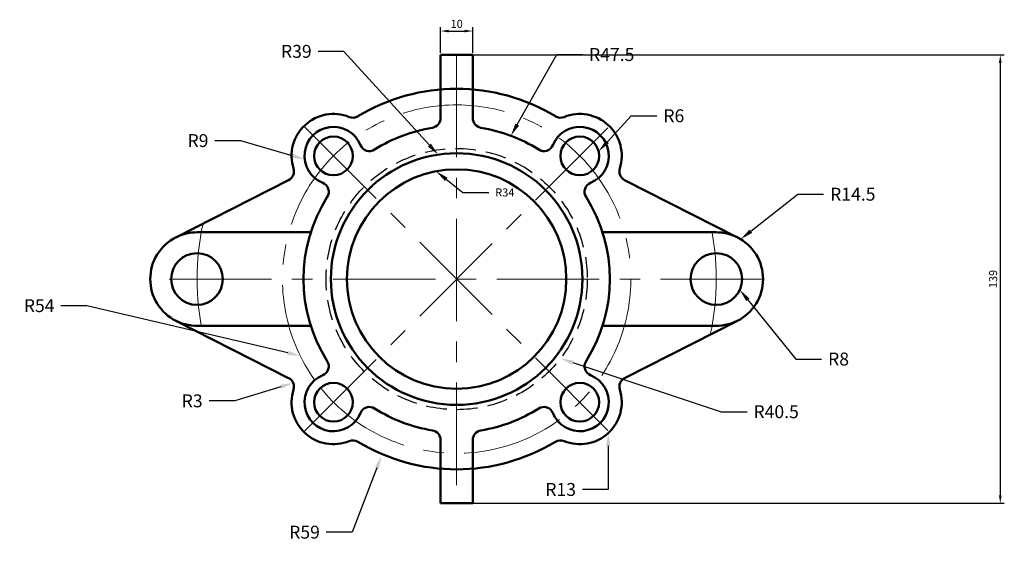
# Model space of a CAD drawing. Units: millimetres. Extents: x 2698 to 3004, y 1503 to 1665.
import ezdxf
from ezdxf import colors
from ezdxf.entities.mleader import LeaderData, LeaderLine
from ezdxf.math import Vec2, Vec3

# ---------------------------------------------------------------- set-up
doc = ezdxf.new("R2010")
doc.units = ezdxf.units.MM
doc.linetypes.add('CENTER', pattern=[50.8, 31.75, -6.35, 6.35, -6.35])
doc.linetypes.add('HIDDEN', pattern=[9.525, 6.35, -3.175])
for name, color, linetype, lineweight in [('M-CNTR', 4, 'CENTER', 18), ('M-DIMS', 2, 'Continuous', 25), ('M-HIDN', 1, 'HIDDEN', 25), ('M-OUTL', 7, 'Continuous', 50), ('M-TEXT', 3, 'Continuous', 25)]:
    doc.layers.add(name, color=color, linetype=linetype, lineweight=lineweight)
doc.styles.get("Standard").update_dxf_attribs({"font": 'arial.ttf'})
doc.dimstyles.new('ISO-25', dxfattribs={"dimtxt": 2.5, "dimasz": 2.5, "dimexe": 1.25, "dimexo": 0.625, "dimtad": 1, "dimtxsty": 'Standard', "dimcen": 2.5, "dimadec": 0, "dimazin": 0, "dimtfac": 1, "dimtmove": 0, "dimatfit": 3, "dimfxl": 1, "dimarcsym": 0})

# ---------------------------------------------------------------- blocks, each defined once
blk = doc.blocks.new('*D1')
at = {"layer": 'Defpoints', "color": 0, "transparency": 16777216}
for p in [(2838.92, 1661.31), (2828.92, 1653.93), (2838.92, 1653.93)]:
    blk.add_point(p, dxfattribs=at)
at = {"layer": 'M-DIMS', "color": 0, "lineweight": -2, "transparency": 16777216}
for p, q in [((2828.92, 1654.55), (2828.92, 1662.56)), ((2831.42, 1661.31), (2836.42, 1661.31)), ((2838.92, 1654.55), (2838.92, 1662.56))]:
    blk.add_line(p, q, dxfattribs=at)
at = {"layer": 'M-DIMS', "color": 0, "transparency": 16777216}
for points in [[(2831.42, 1661.72), (2831.42, 1660.89), (2828.92, 1661.31)], [(2836.42, 1661.72), (2836.42, 1660.89), (2838.92, 1661.31)]]:
    blk.add_solid(points, dxfattribs=at)
at = {"layer": 'M-DIMS', "color": 0, "transparency": 16777216, "insert": (2833.92, 1663.21), "char_height": 2.5, "attachment_point": 5}
blk.add_mtext('10', dxfattribs=at)
blk = doc.blocks.new('*D2')
at = {"layer": 'Defpoints', "color": 0, "transparency": 16777216}
for p in [(2833.92, 1653.93), (2833.92, 1514.93), (3002.46, 1514.93)]:
    blk.add_point(p, dxfattribs=at)
at = {"layer": 'M-DIMS', "color": 0, "lineweight": -2, "transparency": 16777216}
for p, q in [((2834.54, 1653.93), (3003.71, 1653.93)), ((3002.46, 1651.43), (3002.46, 1517.43)), ((2834.54, 1514.93), (3003.71, 1514.93))]:
    blk.add_line(p, q, dxfattribs=at)
at = {"layer": 'M-DIMS', "color": 0, "transparency": 16777216}
for points in [[(3002.04, 1651.43), (3002.87, 1651.43), (3002.46, 1653.93)], [(3002.04, 1517.43), (3002.87, 1517.43), (3002.46, 1514.93)]]:
    blk.add_solid(points, dxfattribs=at)
at = {"layer": 'M-DIMS', "color": 0, "transparency": 16777216, "insert": (3000.56, 1584.43), "char_height": 2.5, "attachment_point": 5, "rotation": 90}
blk.add_mtext('139', dxfattribs=at)
blk = doc.blocks.new('BOLT-HOLE-LUG')
blk.add_circle((12.73, 8.61), 6)
blk.add_arc((12.73, 8.61), 9, 21.8384, 248.1616)

msp = doc.modelspace()

# ---------------------------------------------------------------- linework, layer by layer
at = {"layer": 'M-CNTR'}
for p, q in [((2833.916, 1653.928), (2833.916, 1514.928)), ((2786.54, 1537.052), (2881.292, 1631.804)), ((2786.54, 1631.804), (2881.292, 1537.052)), ((2928.916, 1584.428), (2738.916, 1584.428))]:
    msp.add_line(p, q, dxfattribs=at)
for radius, start, end in [(54, 218.63053, 215.43962), (80.5, 167.65726, 192.34274), (80.5, 347.65726, 12.34274)]:
    msp.add_arc((2833.916, 1584.428), radius, start, end, dxfattribs=at)
at = {"layer": 'M-HIDN'}
msp.add_circle((2833.916, 1584.428), 40.5, dxfattribs=at)
at = {"layer": 'M-OUTL'}
for p, q in [((2828.916, 1653.928), (2838.916, 1653.928)), ((2828.916, 1634.29), (2828.916, 1653.928)), ((2838.916, 1653.928), (2838.916, 1634.29)), ((2746.85, 1597.356), (2781.832, 1615.122)), ((2920.982, 1597.356), (2886, 1615.122)), ((2753.416, 1598.928), (2788.683, 1598.928)), ((2879.149, 1598.928), (2914.416, 1598.928)), ((2746.85, 1571.499), (2781.832, 1553.734)), ((2753.416, 1569.928), (2788.683, 1569.928)), ((2879.149, 1569.928), (2914.416, 1569.928)), ((2920.982, 1571.499), (2886, 1553.734)), ((2828.916, 1534.565), (2828.916, 1514.928)), ((2838.916, 1534.565), (2838.916, 1514.928)), ((2838.916, 1514.928), (2828.916, 1514.928))]:
    msp.add_line(p, q, dxfattribs=at)
for centre, radius in [((2833.916, 1584.428), 39), ((2833.916, 1584.428), 34), ((2753.416, 1584.428), 8), ((2914.416, 1584.428), 8)]:
    msp.add_circle(centre, radius, dxfattribs=at)
for centre, radius, start, end in [((2833.916, 1584.428), 59, 58.75383, 121.24617), ((2795.732, 1622.612), 13, 67.88538, 197.51435), ((2801.756, 1637.434), 3, 247.88538, 301.24617), ((2825.916, 1634.29), 3, 279.11496, 0), ((2841.916, 1634.29), 3, 180, 260.88504), ((2866.076, 1637.434), 3, 238.75383, 292.11462), ((2872.1, 1622.612), 13, 342.48565, 112.11462), ((2833.916, 1584.428), 47.5, 99.11496, 122.38075), ((2833.916, 1584.428), 47.5, 57.61925, 80.88504), ((2806.871, 1627.075), 3, 201.83841, 302.38075), ((2860.961, 1627.075), 3, 237.61925, 338.16159), ((2780.474, 1617.796), 3, 296.92354, 17.51435), ((2887.358, 1617.796), 3, 162.48565, 243.07646), ((2791.268, 1611.473), 3, 327.61925, 68.16159), ((2876.564, 1611.473), 3, 111.83841, 212.38075), ((2833.916, 1584.428), 47.5, 147.61925, 212.38075), ((2833.916, 1584.428), 47.5, 327.61925, 32.38075), ((2753.416, 1584.428), 14.5, 84.83282, 275.16718), ((2914.416, 1584.428), 14.5, 264.83282, 95.16718), ((2791.268, 1557.383), 3, 291.83841, 32.38075), ((2876.564, 1557.383), 3, 147.61925, 248.16159), ((2780.474, 1551.059), 3, 342.48565, 63.07646), ((2887.358, 1551.059), 3, 116.92354, 197.51435), ((2795.732, 1546.244), 13, 162.48565, 292.11462), ((2872.1, 1546.244), 13, 247.88538, 17.51435), ((2806.871, 1541.78), 3, 57.61925, 158.16159), ((2860.961, 1541.78), 3, 21.83841, 122.38075), ((2833.916, 1584.428), 47.5, 237.61925, 260.88504), ((2833.916, 1584.428), 47.5, 279.11496, 302.38075), ((2825.916, 1534.565), 3, 0, 80.88504), ((2841.916, 1534.565), 3, 99.11496, 180), ((2801.756, 1531.421), 3, 58.75383, 112.11462), ((2833.916, 1584.428), 59, 238.75383, 301.24617), ((2866.076, 1531.421), 3, 67.88538, 121.24617)]:
    msp.add_arc(centre, radius, start, end, dxfattribs=at)

# ---------------------------------------------------------------- block references
msp.add_blockref('BOLT-HOLE-LUG', (2783, 1614), dxfattribs=at)
for p, rotation in [((2863.488, 1635.344), 270.0000000000005), ((2804.344, 1533.512), 90.00000000000315), ((2884.832, 1554.856), 180)]:
    msp.add_blockref('BOLT-HOLE-LUG', p, dxfattribs=dict(at, rotation=rotation))

# ---------------------------------------------------------------- dimensions: what is measured, and where the dimension line sits
at = {"layer": 'M-DIMS'}
dim = msp.add_linear_dim(base=(2838.916, 1661.307), p1=(2828.916, 1653.928), p2=(2838.916, 1653.928), dimstyle='ISO-25', override={"dimclrd": 0, "dimclre": 0, "dimclrt": 0}, dxfattribs=at)
dim.commit()
dim.dimension.update_dxf_attribs({"geometry": '*D1', "text_midpoint": (2833.916, 1663.209)})
dim = msp.add_linear_dim(base=(3002.458, 1514.928), p1=(2833.916, 1653.928), p2=(2833.916, 1514.928), angle=90, dimstyle='ISO-25', override={"dimclrd": 0, "dimclre": 0, "dimclrt": 0}, dxfattribs=at)
dim.commit()
dim.dimension.update_dxf_attribs({"geometry": '*D2', "text_midpoint": (3000.556, 1584.428)})

# ---------------------------------------------------------------- leaders
at = {"layer": 'M-TEXT'}
ml = msp.add_multileader_mtext('Standard', dxfattribs=at)
ml.set_content('R39', color=256)
ml.set_leader_properties()
ml.build(insert=Vec2(0, 0))
ctx = ml.context
ctx.base_point, ctx.plane_origin = Vec3(2777.405, 1654.98), Vec3(2828.164, 1623.001)
ctx.text_align_type = 2
notes = []
notes.append((ctx, [(0, (1, 1, 0), (2798.972, 1654.98), (-1, 0), 8, [(0, [(2828.164, 1623.001)], 0, [])])]))
ctx.mtext.insert, ctx.mtext.alignment, ctx.mtext.flow_direction = Vec3(2788.972, 1657.015), 3, 5
ml = msp.add_multileader_mtext('Standard', dxfattribs=at)
ml.set_content('R47.5', color=256)
ml.set_leader_properties()
ml.build(insert=Vec2(0, 0))
ctx = ml.context
ctx.base_point, ctx.plane_origin = Vec3(2872.956, 1653.993), Vec3(2850.743, 1628.847)
notes.append((ctx, [(0, (1, 1, 0), (2864.956, 1653.993), (1, 0), 8, [(0, [(2850.743, 1628.847)], 0, [])])]))
ctx.mtext.insert, ctx.mtext.flow_direction = Vec3(2874.956, 1656.027), 5
ml = msp.add_multileader_mtext('Standard', dxfattribs=at)
ml.set_content('R6', color=256)
ml.set_leader_properties()
ml.build(insert=Vec2(0, 0))
ctx = ml.context
ctx.base_point, ctx.plane_origin = Vec3(2896, 1635.013), Vec3(2877.935, 1624.008)
notes.append((ctx, [(0, (1, 1, 0), (2888, 1635.013), (1, 0), 8, [(0, [(2877.935, 1624.008)], 0, [])])]))
ctx.mtext.insert, ctx.mtext.flow_direction = Vec3(2898, 1637.047), 5
ml = msp.add_multileader_mtext('Standard', dxfattribs=at)
ml.set_content('R9', color=256)
ml.set_leader_properties()
ml.build(insert=Vec2(0, 0))
ctx = ml.context
ctx.base_point, ctx.plane_origin = Vec3(2748.509, 1627.319), Vec3(2786.796, 1621.538)
ctx.text_align_type = 2
notes.append((ctx, [(0, (1, 1, 0), (2766.968, 1627.319), (-1, 0), 8, [(0, [(2786.796, 1621.538)], 0, [])])]))
ctx.mtext.insert, ctx.mtext.alignment, ctx.mtext.flow_direction = Vec3(2756.968, 1629.353), 3, 5
ml = msp.add_multileader_mtext('Standard', dxfattribs=at)
ml.set_content('R34', color=256)
ml.set_leader_properties()
ml.build(insert=Vec2(0, 0))
ctx = ml.context
ctx.base_point, ctx.char_height, ctx.plane_origin = Vec3(2843.883, 1611.259), 2.5, Vec3(2827.54, 1617.825)
notes.append((ctx, [(0, (1, 1, 0), (2835.883, 1611.259), (1, 0), 8, [(0, [(2827.54, 1617.825)], 0, [])])]))
ctx.mtext.insert, ctx.mtext.width, ctx.mtext.flow_direction = Vec3(2845.883, 1612.532), 4.67791, 5
ml = msp.add_multileader_mtext('Standard', dxfattribs=at)
ml.set_content('R14.5', color=256)
ml.set_leader_properties()
ml.build(insert=Vec2(0, 0))
ctx = ml.context
ctx.base_point, ctx.plane_origin = Vec3(2947.7, 1610.693), Vec3(2921.991, 1596.792)
notes.append((ctx, [(0, (1, 1, 0), (2939.7, 1610.693), (1, 0), 8, [(0, [(2921.991, 1596.792)], 0, [])])]))
ctx.mtext.insert, ctx.mtext.flow_direction = Vec3(2949.7, 1612.727), 5
ml = msp.add_multileader_mtext('Standard', dxfattribs=at)
ml.set_content('R8', color=256)
ml.set_leader_properties()
ml.build(insert=Vec2(0, 0))
ctx = ml.context
ctx.base_point, ctx.plane_origin = Vec3(2947.069, 1559.6), Vec3(2921.691, 1581.101)
notes.append((ctx, [(0, (1, 1, 0), (2939.069, 1559.6), (1, 0), 8, [(0, [(2921.691, 1581.101)], 0, [])])]))
ctx.mtext.insert, ctx.mtext.flow_direction = Vec3(2949.069, 1561.635), 5
ml = msp.add_multileader_mtext('Standard', dxfattribs=at)
ml.set_content('R54', color=256)
ml.set_leader_properties()
ml.build(insert=Vec2(0, 0))
ctx = ml.context
ctx.base_point, ctx.plane_origin = Vec3(2697.696, 1576.153), Vec3(2785.452, 1560.61)
ctx.text_align_type = 2
notes.append((ctx, [(0, (1, 1, 0), (2719.238, 1576.153), (-1, 0), 8, [(0, [(2785.452, 1560.61)], 0, [])])]))
ctx.mtext.insert, ctx.mtext.alignment, ctx.mtext.flow_direction = Vec3(2709.238, 1578.188), 3, 5
ml = msp.add_multileader_mtext('Standard', dxfattribs=at)
ml.set_content('R40.5', color=256)
ml.set_leader_properties()
ml.build(insert=Vec2(0, 0))
ctx = ml.context
ctx.base_point, ctx.plane_origin = Vec3(2923.934, 1543.272), Vec3(2866.091, 1559.83)
notes.append((ctx, [(0, (1, 1, 0), (2915.934, 1543.272), (1, 0), 8, [(0, [(2866.091, 1559.83)], 0, [])])]))
ctx.mtext.insert, ctx.mtext.flow_direction = Vec3(2925.934, 1545.306), 5
ml = msp.add_multileader_mtext('Standard', dxfattribs=at)
ml.set_content('R3', color=256)
ml.set_leader_properties()
ml.build(insert=Vec2(0, 0))
ctx = ml.context
ctx.base_point, ctx.plane_origin = Vec3(2746.711, 1546.632), Vec3(2783.24, 1552.221)
ctx.text_align_type = 2
notes.append((ctx, [(0, (1, 1, 0), (2765.161, 1546.632), (-1, 0), 8, [(0, [(2783.24, 1552.221)], 0, [])])]))
ctx.mtext.insert, ctx.mtext.alignment, ctx.mtext.flow_direction = Vec3(2755.161, 1548.668), 3, 5
ml = msp.add_multileader_mtext('Standard', dxfattribs=at)
ml.set_content('R13', color=256)
ml.set_leader_properties()
ml.build(insert=Vec2(0, 0))
ctx = ml.context
ctx.base_point, ctx.plane_origin = Vec3(2859.358, 1519.171), Vec3(2880.916, 1536.69)
ctx.text_align_type = 2
notes.append((ctx, [(0, (1, 1, 0), (2880.916, 1519.171), (-1, 0), 8, [(0, [(2880.916, 1536.69)], 0, [])])]))
ctx.mtext.insert, ctx.mtext.alignment, ctx.mtext.flow_direction = Vec3(2870.916, 1521.206), 3, 5
ml = msp.add_multileader_mtext('Standard', dxfattribs=at)
ml.set_content('R59', color=256)
ml.set_leader_properties()
ml.build(insert=Vec2(0, 0))
ctx = ml.context
ctx.base_point, ctx.plane_origin = Vec3(2779.946, 1505.929), Vec3(2810.608, 1529.64)
ctx.text_align_type = 2
notes.append((ctx, [(0, (1, 1, 0), (2801.512, 1505.929), (-1, 0), 8, [(0, [(2810.608, 1529.64)], 0, [])])]))
ctx.mtext.insert, ctx.mtext.alignment, ctx.mtext.flow_direction = Vec3(2791.512, 1507.963), 3, 5
for ctx, leaders in notes:
    for number, flags, end, landing, length, lines in leaders:
        leader = LeaderData()
        leader.index, (leader.has_last_leader_line, leader.has_dogleg_vector, leader.attachment_direction) = number, flags
        leader.last_leader_point, leader.dogleg_vector, leader.dogleg_length = Vec3(end), Vec3(landing), length
        for number, points, colour, breaks in lines:
            line = LeaderLine()
            line.index, line.vertices, line.color, line.breaks = number, Vec3.list(points), colors.encode_raw_color(colour), breaks
            leader.lines.append(line)
        ctx.leaders.append(leader)

doc.saveas('drawing.dxf')
